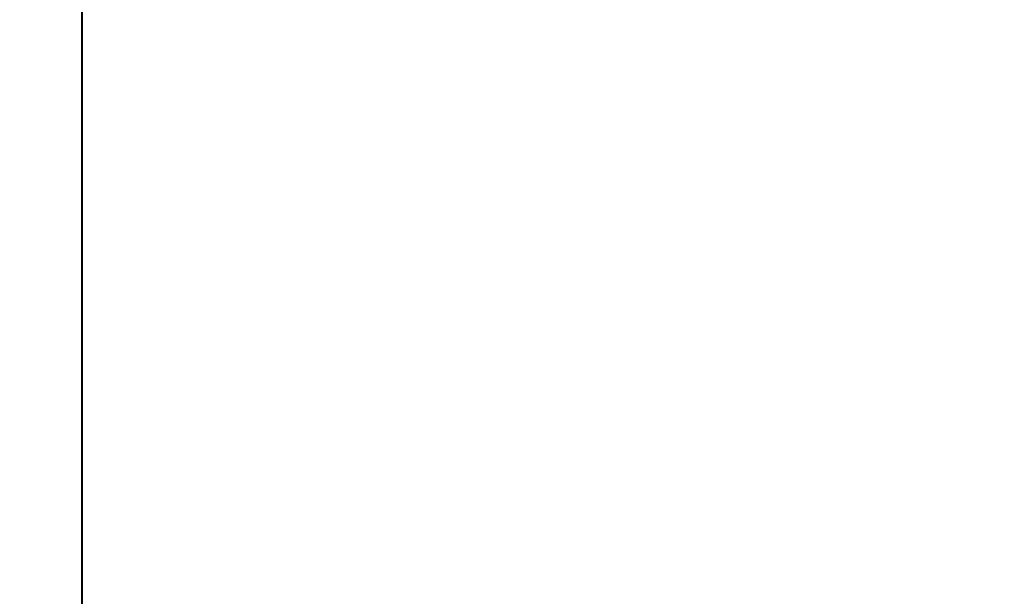
# Model space of a CAD drawing. Units: inches. Extents: x 459864 to 460310, y 324185 to 324787.
# Tile 82 of 112: x 460247.1148819 to 460247.1155894, y 324283.4834181 to 324283.4838323. Entities that reach past the tile are written whole.
import ezdxf

# ---------------------------------------------------------------- set-up
doc = ezdxf.new("R2010")
doc.units = ezdxf.units.IN
doc.layers.add('A-ANNO-DIMS', color=2, linetype='Continuous', lineweight=18)
doc.layers.add('A-WALL', color=7, linetype='Continuous', lineweight=40)
doc.styles.get("Standard").update_dxf_attribs({"font": 'arial.ttf'})
doc.dimstyles.new('ISO-25', dxfattribs={"dimtxt": 6, "dimasz": 2.5, "dimexe": 1.25, "dimexo": 0.625, "dimtad": 1, "dimdec": 1, "dimlunit": 3, "dimtxsty": 'Standard', "dimcen": 2.5, "dimadec": 0, "dimazin": 0, "dimtfac": 1, "dimtdec": 1, "dimtmove": 0, "dimatfit": 3, "dimfxl": 1, "dimarcsym": 0})

# ---------------------------------------------------------------- blocks, each defined once
blk = doc.blocks.new('*D21')
at = {"layer": 'A-ANNO-DIMS', "color": 0, "lineweight": -2, "transparency": 16777216}
for p, q in [((460247.73992657, 324715.48323276), (460309.58036853, 324715.48323276)), ((460308.33036853, 324712.98323276), (460308.33036853, 324285.98323276)), ((460247.73992657, 324283.48323276), (460309.58036853, 324283.48323276))]:
    blk.add_line(p, q, dxfattribs=at)
at = {"layer": 'A-ANNO-DIMS', "color": 0, "transparency": 16777216}
for points in [[(460307.91370186, 324712.98323276), (460308.74703519, 324712.98323276), (460308.33036853, 324715.48323276)], [(460307.91370186, 324285.98323276), (460308.74703519, 324285.98323276), (460308.33036853, 324283.48323276)]]:
    blk.add_solid(points, dxfattribs=at)
at = {"layer": 'Defpoints', "color": 0, "transparency": 16777216}
for p in [(460247.11492657, 324715.48323276), (460247.11492657, 324283.48323276), (460308.33036853, 324283.48323276)]:
    blk.add_point(p, dxfattribs=at)
at = {"layer": 'A-ANNO-DIMS', "color": 0, "transparency": 16777216, "insert": (460304.63988421, 324499.48323276), "char_height": 6, "attachment_point": 5, "rotation": 90}
blk.add_mtext("36'", dxfattribs=at)
blk = doc.blocks.new('*D62')
at = {"layer": 'A-ANNO-DIMS', "color": 0, "lineweight": -2, "transparency": 16777216}
for p, q in [((460247.739927, 324332.73872), (460278.764927, 324332.73872)), ((460277.514927, 324330.23872), (460277.514927, 324285.983233)), ((460247.739927, 324283.483233), (460278.764927, 324283.483233))]:
    blk.add_line(p, q, dxfattribs=at)
at = {"layer": 'A-ANNO-DIMS', "color": 0, "transparency": 16777216}
for points in [[(460277.09826033, 324330.23872), (460277.93159367, 324330.23872), (460277.514927, 324332.73872)], [(460277.09826033, 324285.983233), (460277.93159367, 324285.983233), (460277.514927, 324283.483233)]]:
    blk.add_solid(points, dxfattribs=at)
at = {"layer": 'Defpoints', "color": 0, "transparency": 16777216}
for p in [(460247.114927, 324332.73872), (460247.114927, 324283.483233), (460277.514927, 324283.483233)]:
    blk.add_point(p, dxfattribs=at)
at = {"layer": 'A-ANNO-DIMS', "color": 0, "transparency": 16777216, "insert": (460273.78760776, 324308.1109765), "char_height": 6, "attachment_point": 5, "rotation": 90}
blk.add_mtext('4\'-1 1/2"', dxfattribs=at)
blk = doc.blocks.new('*D67')
at = {"layer": 'A-ANNO-DIMS', "color": 0, "lineweight": -2, "transparency": 16777216}
for p, q in [((460208.114927, 324284.108233), (460208.114927, 324315.133233)), ((460247.114927, 324284.108233), (460247.114927, 324315.133233)), ((460210.614927, 324313.883233), (460244.614927, 324313.883233))]:
    blk.add_line(p, q, dxfattribs=at)
at = {"layer": 'A-ANNO-DIMS', "color": 0, "transparency": 16777216}
for points in [[(460210.614927, 324314.29989967), (460210.614927, 324313.46656633), (460208.114927, 324313.883233)], [(460244.614927, 324314.29989967), (460244.614927, 324313.46656633), (460247.114927, 324313.883233)]]:
    blk.add_solid(points, dxfattribs=at)
at = {"layer": 'Defpoints', "color": 0, "transparency": 16777216}
for p in [(460247.114927, 324313.883233), (460208.114927, 324283.483233), (460247.114927, 324283.483233)]:
    blk.add_point(p, dxfattribs=at)
at = {"layer": 'A-ANNO-DIMS', "color": 0, "transparency": 16777216, "insert": (460227.614927, 324317.57371731), "char_height": 6, "attachment_point": 5}
blk.add_mtext('3\'-3"', dxfattribs=at)

msp = doc.modelspace()

# ---------------------------------------------------------------- linework, layer by layer
at = {"layer": 'A-WALL'}
msp.add_line((460247.11492657, 324470.98323276), (460247.11492657, 324283.48323276), dxfattribs=at)

# ---------------------------------------------------------------- dimensions: what is measured, and where the dimension line sits
at = {"layer": 'A-ANNO-DIMS'}
for base, p1, p2, angle, override, picture, middle in [((460308.33036853, 324283.48323276), (460247.11492657, 324715.48323276), (460247.11492657, 324283.48323276), 90, {"dimclrd": 0, "dimclre": 0, "dimclrt": 0}, '*D21', (460304.63988421, 324499.48323276)), ((460277.514927, 324283.483233), (460247.114927, 324332.73872), (460247.114927, 324283.483233), 270, {"dimdec": 1, "dimlfac": 1, "dimrnd": 0, "dimzin": 1, "dimdsep": 46, "dimlunit": 4, "dimfrac": 2}, '*D62', (460273.78760776, 324308.1109765))]:
    dim = msp.add_linear_dim(base=base, p1=p1, p2=p2, angle=angle, dimstyle='ISO-25', override=override, dxfattribs=at)
    dim.commit()
    dim.dimension.update_dxf_attribs({"geometry": picture, "text_midpoint": middle})
dim = msp.add_linear_dim(base=(460247.114927, 324313.883233), p1=(460208.114927, 324283.483233), p2=(460247.114927, 324283.483233), dimstyle='ISO-25', override={"dimdec": 1, "dimlfac": 1, "dimrnd": 0, "dimzin": 1, "dimdsep": 46, "dimlunit": 4, "dimfrac": 2}, dxfattribs=at)
dim.commit()
dim.dimension.update_dxf_attribs({"geometry": '*D67', "text_midpoint": (460227.614927, 324317.57371731)})

doc.saveas('drawing.dxf')
